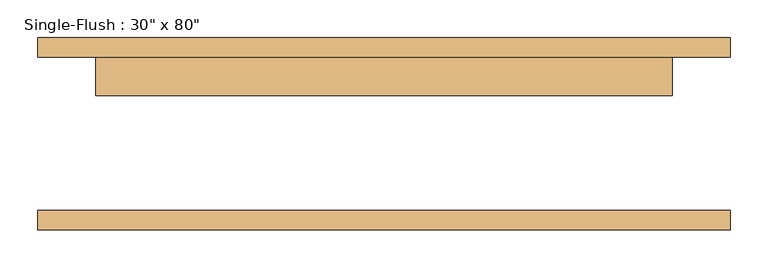
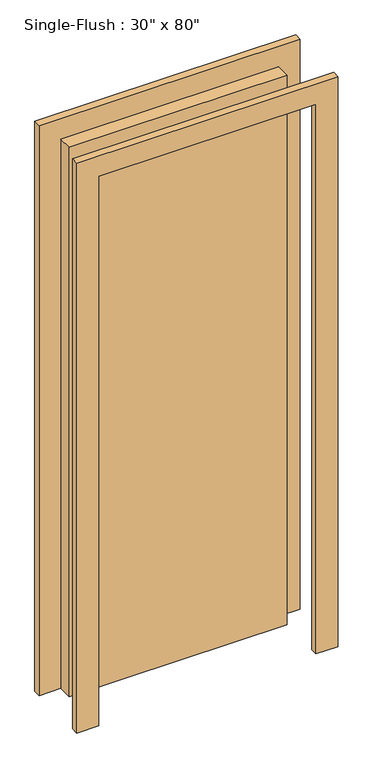
"""IFC4 building model written with IfcOpenShell, lengths in millimetres: door geometry."""

from ifc_helpers import new_model, si_unit, frame, origin, origin_with_axes, place, context, project, spatial, polyline, outline, extrude, source, transform, mapped, element, save


def door_fadea3f2(model_context):
    return source(origin(), model_context, "Body", "SweptSolid", [
        extrude(outline(polyline([(2108.2, -457.2), (0.0, -457.2), (0.0, -381.0), (2032.0, -381.0), (2032.0, 381.0), (0.0, 381.0), (0.0, 457.2), (2108.2, 457.2), (2108.2, -457.2)])), frame((0.0, 101.6, 0.0), z_axis=(0.0, 1.0, 0.0), x_axis=(0.0, 0.0, 1.0)), (0.0, 0.0, 1.0), 25.4),
        extrude(outline(polyline([(2108.2, 457.2), (2108.2, -457.2), (0.0, -457.2), (0.0, -381.0), (2032.0, -381.0), (2032.0, 381.0), (0.0, 381.0), (0.0, 457.2), (2108.2, 457.2)])), frame((0.0, -127.0, 0.0), z_axis=(0.0, 1.0, 0.0), x_axis=(0.0, 0.0, 1.0)), (0.0, 0.0, 1.0), 25.4),
        extrude(outline(polyline([(381.0, 50.8), (-381.0, 50.8), (-381.0, 101.6), (381.0, 101.6), (381.0, 50.8)])), origin_with_axes(), (0.0, 0.0, 1.0), 2032.0),
    ])


if __name__ == "__main__":
    model = new_model("IFC4")
    model_context = context("Model", 3, world=origin())
    ifc_project = project(units=[si_unit("LENGTHUNIT", "METRE", prefix="MILLI")], contexts=[model_context])
    site = spatial("IfcSite", under=ifc_project)
    building = spatial("IfcBuilding", under=site)
    placement = place(None, origin())
    door_shape = door_fadea3f2(model_context)
    element("IfcDoor", 1, ObjectType="Single-Flush : 30\" x 80\"", at=placement, inside=building, context=model_context, shape_type="MappedRepresentation", body=[
        mapped(door_shape, transform((0.0, 0.0, 0.0), x_axis=(1.0, 0.0, 0.0), y_axis=(0.0, 1.0, 0.0), z_axis=(0.0, 0.0, 1.0))),
    ])
    save(model, "model.ifc")

# Revit data of these elements
# Type "Single-Flush : 30\" x 80\""
#   Type Mark = "5"
#   Assembly Code = "C1020"
#   Thickness = 0' - 2"
#   Height = 6' - 8"
#   Trim Projection Ext = 0' - 1"
#   Trim Projection Int = 0' - 1"
#   Trim Width = 0' - 3"
#   Width = 2' - 6"
#   Door Material = Door - Panel
#   Frame Material = Door - Frame
#   Function = (empty or 0)
#   Wall Closure = (empty or 0)
# Element 1 (IfcDoor, "Single-Flush : 30\" x 80\"")
#   Materials on its faces: "Door - Frame", "Door - Panel"
# Materials
#   "Door - Panel": class "Wood", colour RGB 114 82 51, transparency 0
#   "Door - Frame": colour RGB 153 76 43, transparency 0
